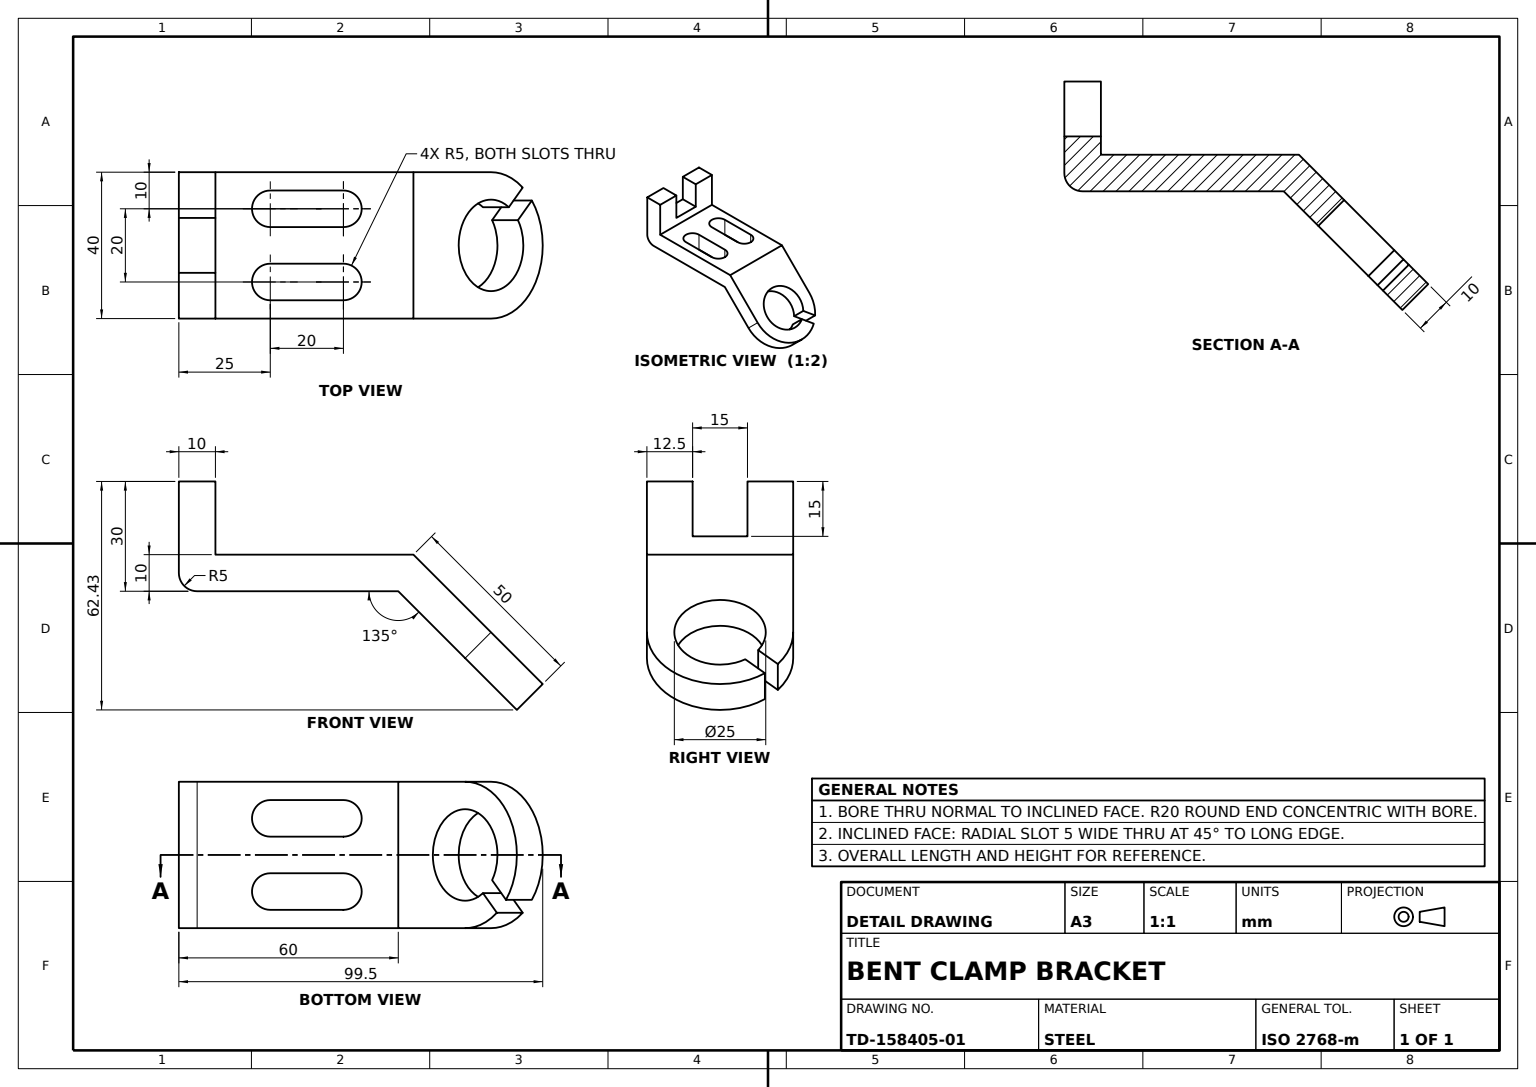
SolidWorks part; units mm, degrees
material "Plain Carbon Steel"
ref_plane "Front Plane" through (0, 0, 0) normal (0, 0, 1) x (1, 0, 0)
ref_plane "Top Plane" through (0, 0, 0) normal (0, 1, 0) x (1, 0, 0)
ref_plane "Right Plane" through (0, 0, 0) normal (1, 0, 0) x (0, 0, -1)
sketch "Bracket Profile Sketch" plane through (0, 0, 0) normal (0, 0, 1) x (1, 0, 0)
  line L0 (0, 5) -> (0, 30)
  line L1 (0, 30) -> (-10, 30)
  line L2 (-10, 30) -> (-10, 10)
  line L3 (-10, 10) -> (-64.1421, 10)
  line L4 (-64.1421, 10) -> (-85.3553, -11.2132)
  line L5 (-85.3553, -11.2132) -> (-78.2843, -18.2843)
  line L6 (-78.2843, -18.2843) -> (-60, 0)
  line L7 (-60, 0) -> (-5, 0)
  line L8 (-60, -1.2433) -> (-60, 0) construction
  line L9 (-60, 0) -> (-60, -24.3215) construction
  arc A0 (0, 5) -> (-5, 0) centre (-5, 5) cw
  point P12 (0, 0)
  dimension "D6" = 5
  dimension "D1" = 10
  dimension "D2" = 60
  dimension "D3" = 30
  dimension "D4" = 10
  dimension "D5" = 20
  dimension "D7" = 135
  dimension "D8" = 10
extrude "Angled Bracket Body" add sketch "Bracket Profile Sketch" along normal mid plane 40
sketch "Guide Upright Sketch" plane through (-37.0711, 37.0711, 0) normal (-0.7071, 0.7071, 0) x (0, 0, 1)
  line L0 (20, -68.2843) -> (-20, -68.2843) construction
  line L1 (20, -38.2843) -> (20, -68.2843) construction
  line L2 (-20, -38.2843) -> (-20, -68.2843) construction
  line L3 (-20, -68.2843) -> (20, -68.2843)
  arc A0 (-20, -68.2843) -> (20, -68.2843) centre (0, -68.2843) ccw
extrude "Guide Upright Boss" add sketch "Guide Upright Sketch" against normal blind 10
sketch "Guide Notch Sketch" plane through (-10, 0, 0) normal (-1, 0, 0) x (0, 0, 1)
  line L0 (20, 30) -> (-20, 30) construction
  line L1 (-7.5, 30) -> (7.5, 30)
  line L2 (-7.5, 30) -> (-7.5, 15)
  line L3 (-7.5, 15) -> (7.5, 15)
  line L4 (7.5, 30) -> (7.5, 15)
  point P6 (0, 15)
  dimension "D1" = 15
  dimension "D2" = 15
extrude "Guide Notch 15x15" cut sketch "Guide Notch Sketch" against normal up to next
sketch "Guide Slots Sketch" plane through (0, 10, 0) normal (0, 1, 0) x (1, 0, 0)
  line L0 (-45, 10) -> (-25, 10) construction
  line L1 (-45, 15) -> (-25, 15)
  line L2 (-45, 5) -> (-25, 5)
  line L3 (0, 0) -> (-34.3444, 0) construction
  line L4 (-10, 7.5) -> (-10, 20) construction
  line L5 (-45, -10) -> (-25, -10) construction
  line L6 (-45, -15) -> (-25, -15)
  line L7 (-45, -5) -> (-25, -5)
  arc A0 (-45, 15) -> (-45, 5) centre (-45, 10) ccw
  arc A1 (-25, 5) -> (-25, 15) centre (-25, 10) ccw
  arc A2 (-45, -15) -> (-45, -5) centre (-45, -10) cw
  arc A3 (-25, -5) -> (-25, -15) centre (-25, -10) cw
  point P2 (-35, 10)
  point P14 (-35, -10)
  dimension "D1" = 20
  dimension "D2" = 15
  dimension "D3" = 10
  dimension "D4" = 10
extrude "Guide Slots" cut sketch "Guide Slots Sketch" against normal up to next
sketch "Angled Trim Sketch" plane through (-37.0711, 37.0711, 0) normal (-0.7071, 0.7071, 0) x (0, 0, 1)
  line L0 (0, -68.2843) -> (0, -91.0461) construction
  line L1 (0, -68.2843) -> (18.0409, -86.3251) construction
  line L2 (6.8925, -78.7123) -> (12.919, -84.7388)
  line L3 (10.428, -75.1768) -> (16.464, -81.2128)
  line L4 (12.919, -84.7388) -> (16.464, -81.2128)
  arc A0 (10.428, -75.1768) -> (6.8925, -78.7123) centre (0, -68.2843) ccw
  dimension "D1" = 25
  dimension "D2" = 45
  dimension "D3" = 5
  dimension "D4" = 32.919
  dimension "D5" = 36.464
extrude "Angled Trim Cut 45deg" cut sketch "Angled Trim Sketch" against normal through all
